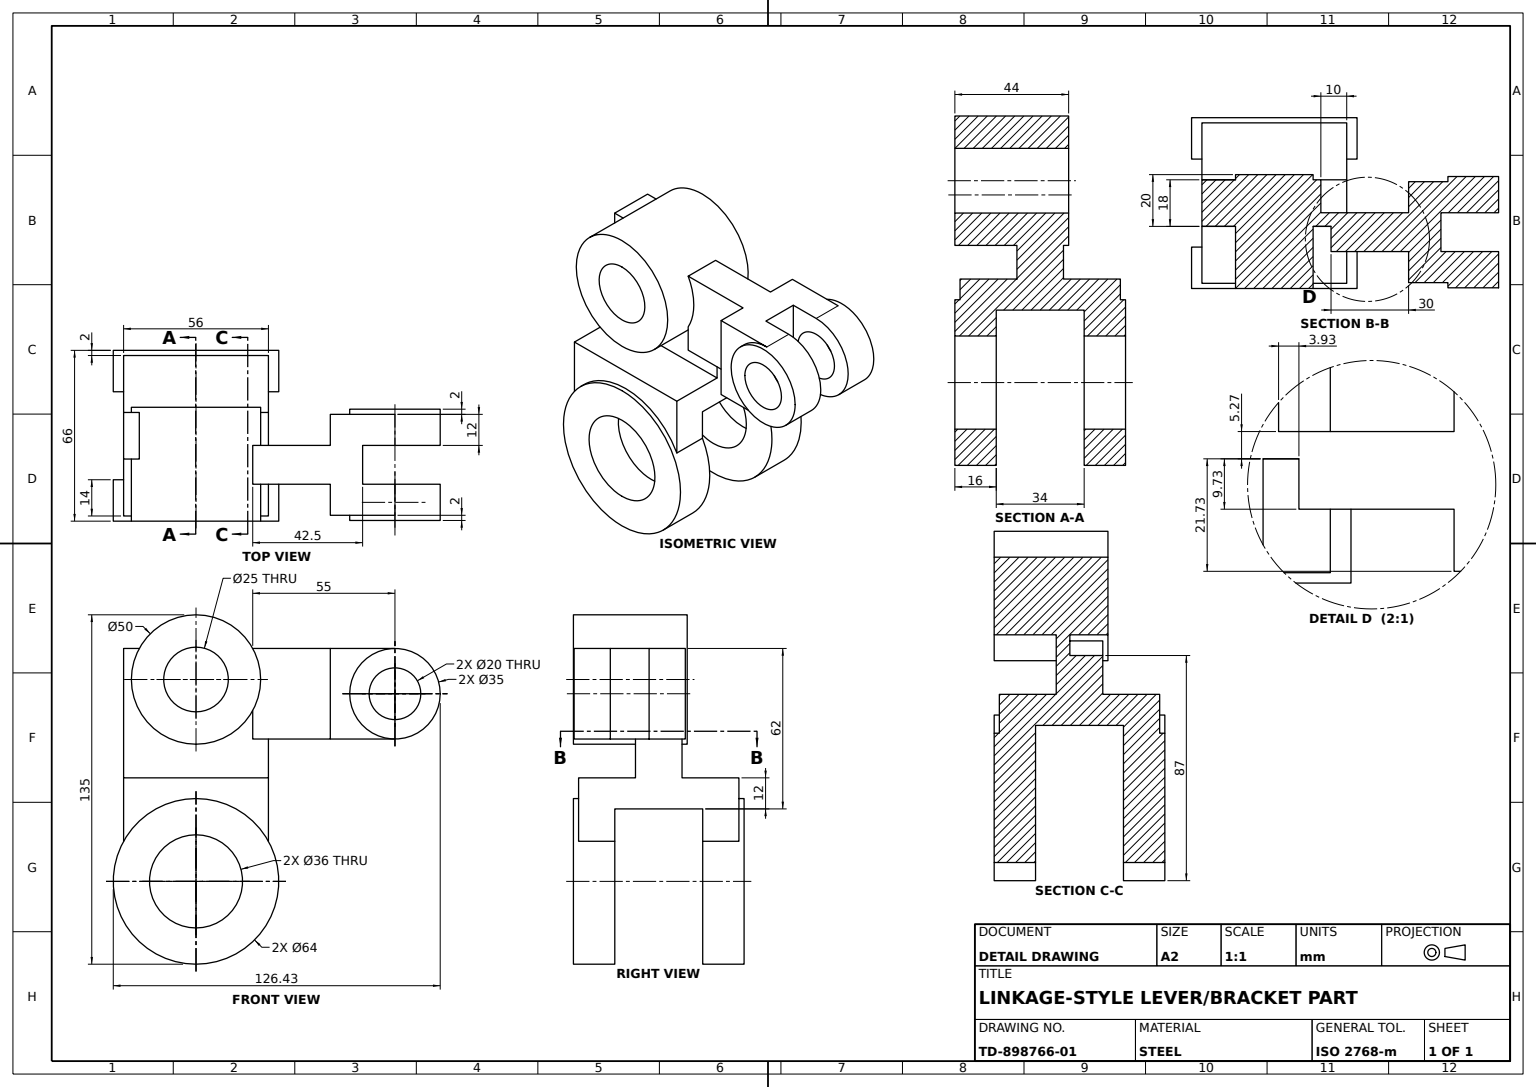
from build123d import *

# Parameters (mm, degrees)
BRACKET_BODY_DEPTH      = 56
SLOT_SKETCH_W           = 62
SLOT_SKETCH_H           = 20
SLOT_CUT_DEPTH          = 90.112288715
LUG_A_SKETCH_R          = 32
LUG_A_SKETCH_R_2        = 18
LUG_A_14MM_DEPTH        = 14
SPACER_START            = 2
SPACER_A_SKETCH_R       = 32
SPACER_A_SKETCH_R_2     = 18
SPACER_A_2MM_DEPTH      = 2
HOLE_A_SKETCH_R         = 18
HOLE_A_DEPTH            = 107.244999882
SPACER_B_SKETCH_R       = 32
SPACER_B_SKETCH_R_2     = 18
SPACER_B_2MM_DEPTH      = 2
LUG_B_SKETCH_R          = 32
LUG_B_SKETCH_R_2        = 18
LUG_B_14MM_DEPTH        = 14
PAD_SKETCH_R            = 25
PAD_SKETCH_R_2          = 12.5
PAD_2MM_DEPTH           = 2
HUB_START               = -44
HUB_SKETCH_R            = 25
HUB_SKETCH_R_2          = 12.5
HUB_44MM_DEPTH          = 44
HUB_BORE_SKETCH_R       = 12.5
HUB_BORE_DEPTH          = 44
ARM_35MM_DEPTH          = 35
ARM_SPACER_A_SKETCH_R   = 17.5
ARM_SPACER_A_SKETCH_R_2 = 10
ARM_SPACER_A_2MM_DEPTH  = 2
ARM_START               = -12
ARM_LUG_SKETCH_R        = 17.5
ARM_LUG_SKETCH_R_2      = 10
ARM_LUG_12MM_DEPTH      = 12
ARM_HOLE_SKETCH_R       = 10
ARM_HOLE_DEPTH          = 150.390672563
ARM_SPACER_B_SKETCH_R   = 17.5
ARM_SPACER_B_SKETCH_R_2 = 10
ARM_SPACER_B_2MM_DEPTH  = 2
ARM_START_2             = -14
ARM_EYE_SKETCH_R        = 17.5
ARM_EYE_SKETCH_R_2      = 10
ARM_EYE_14MM_DEPTH      = 14
ARM_SLOT_SKETCH_W       = 12.731987003
ARM_SLOT_SKETCH_H       = 35
ARM_SLOT_10MM_DEPTH     = 10
PIN_START               = -16
PIN_BOSS_SKETCH_R       = 25
PIN_BOSS_16MM_DEPTH     = 16
PIN_BOSS_HOLE_SKETCH_R  = 12.5
PIN_BOSS_HOLE_DEPTH     = 151.168319402


with BuildPart() as part:
    # Bracket Profile Sketch → Bracket Body (new body)
    with BuildSketch(Plane.XY):
        Polygon((0, 0), (17, 0), (17, -48), (31, -48), (31, 12), (9, 12), (9, 62), (-9, 62), (-9, 12), (-31, 12), (-31, -48), (-17, -48), (-17, 0), align=None)
    extrude(amount=-BRACKET_BODY_DEPTH)

    # Slot Sketch → Slot Cut (cut, through all)
    with BuildSketch(Plane.XY):
        with Locations((0, -38)):
            Rectangle(SLOT_SKETCH_W, SLOT_SKETCH_H)
    extrude(amount=-SLOT_CUT_DEPTH, mode=Mode.SUBTRACT)

    # Lug A Sketch → Lug A 14mm (add)
    with BuildSketch(Plane(origin=(31, 0, 0), x_dir=(0, 0, -1), z_dir=(1, 0, 0))):
        with Locations((28, -28)):
            Circle(LUG_A_SKETCH_R)
        with Locations((28, -28)):
            Circle(LUG_A_SKETCH_R_2, mode=Mode.SUBTRACT)
    extrude(amount=-LUG_A_14MM_DEPTH)

    # Spacer A Sketch → Spacer A 2mm (add)
    with BuildSketch(Plane(origin=(31, 0, 0), x_dir=(0, 0, -1), z_dir=(1, 0, 0)).offset(SPACER_START)):
        with Locations(Location((28, -28, 0), (0, 0, 90))):
            Circle(SPACER_A_SKETCH_R)
        with Locations(Location((28, -28, 0), (0, 0, 90))):
            Circle(SPACER_A_SKETCH_R_2, mode=Mode.SUBTRACT)
    extrude(amount=-SPACER_A_2MM_DEPTH)

    # Hole A Sketch → Hole A (cut, through all)
    with BuildSketch(Plane(origin=(31, 0, 0), x_dir=(0, 0, -1), z_dir=(1, 0, 0))):
        with Locations(Location((28, -28, 0), (0, 0, 90))):
            Circle(HOLE_A_SKETCH_R)
    extrude(amount=-HOLE_A_DEPTH, mode=Mode.SUBTRACT)

    # Spacer B Sketch → Spacer B 2mm (add)
    with BuildSketch(Plane.ZY.offset(31)):
        with Locations(Location((-28, -28, 0), (0, 0, 90))):
            Circle(SPACER_B_SKETCH_R)
        with Locations(Location((-28, -28, 0), (0, 0, 90))):
            Circle(SPACER_B_SKETCH_R_2, mode=Mode.SUBTRACT)
    extrude(amount=SPACER_B_2MM_DEPTH)

    # Lug B Sketch → Lug B 14mm (add)
    with BuildSketch(Plane(origin=(-17, 0, 0), x_dir=(0, 0, -1), z_dir=(1, 0, 0))):
        with Locations(Location((28, -28, 0), (0, 0, 90))):
            Circle(LUG_B_SKETCH_R)
        with Locations(Location((28, -28, 0), (0, 0, 90))):
            Circle(LUG_B_SKETCH_R_2, mode=Mode.SUBTRACT)
    extrude(amount=-LUG_B_14MM_DEPTH)

    # Pad Sketch → Pad 2mm (add)
    with BuildSketch(Plane.ZY.offset(9)):
        with Locations(Location((-28, 50, 0), (0, 0, 151.314597986))):
            Circle(PAD_SKETCH_R)
        with Locations(Location((-28, 50, 0), (0, 0, 73.739795292))):
            Circle(PAD_SKETCH_R_2, mode=Mode.SUBTRACT)
    extrude(amount=PAD_2MM_DEPTH)

    # Hub Sketch → Hub 44mm (add)
    with BuildSketch(Plane.ZY.offset(11).offset(HUB_START)):
        with Locations(Location((-28, 50, 0), (0, 0, 270))):
            Circle(HUB_SKETCH_R)
        with Locations(Location((-28, 50, 0), (0, 0, 270))):
            Circle(HUB_SKETCH_R_2, mode=Mode.SUBTRACT)
    extrude(amount=HUB_44MM_DEPTH)

    # Hub Bore Sketch → Hub Bore (cut)
    with BuildSketch(Plane.ZY.offset(9).offset(HUB_START)):
        with Locations(Location((-28, 50, 0), (0, 0, 270))):
            Circle(HUB_BORE_SKETCH_R)
    extrude(amount=HUB_BORE_DEPTH, mode=Mode.SUBTRACT)

    # Arm Profile Sketch → Arm 35mm (add)
    with BuildSketch(Plane(origin=(0, 62, 0), x_dir=(1, 0, 0), z_dir=(0, 1, 0))):
        Polygon((3.731987003, 49.931712199), (3.731987003, 79.931712199), (-8.268012997, 79.931712199), (-8.268012997, 104.931712199), (3.731987003, 104.931712199), (3.731987003, 92.431712199), (18.731987003, 92.431712199), (18.731987003, 104.931712199), (30.731987003, 104.931712199), (30.731987003, 79.931712199), (18.731987003, 79.931712199), (18.731987003, 49.931712199), align=None)
    extrude(amount=-ARM_35MM_DEPTH)

    # Arm Spacer A Sketch → Arm Spacer A 2mm (add)
    with BuildSketch(Plane.ZY.offset(8.268012997)):
        with Locations(Location((-104.931712199, 44.5, 0), (0, 0, 270))):
            Circle(ARM_SPACER_A_SKETCH_R)
        with Locations(Location((-104.931712199, 44.5, 0), (0, 0, 90))):
            Circle(ARM_SPACER_A_SKETCH_R_2, mode=Mode.SUBTRACT)
    extrude(amount=ARM_SPACER_A_2MM_DEPTH)

    # Arm Lug Sketch → Arm Lug 12mm (add)
    with BuildSketch(Plane.ZY.offset(8.268012997).offset(ARM_START)):
        with Locations(Location((-104.931712199, 44.5, 0), (0, 0, 90))):
            Circle(ARM_LUG_SKETCH_R)
        with Locations(Location((-104.931712199, 44.5, 0), (0, 0, 90))):
            Circle(ARM_LUG_SKETCH_R_2, mode=Mode.SUBTRACT)
    extrude(amount=ARM_LUG_12MM_DEPTH)

    # Arm Hole Sketch → Arm Hole (cut, through all)
    with BuildSketch(Plane.ZY.offset(8.268012997)):
        with Locations((-104.931712199, 44.5)):
            Circle(ARM_HOLE_SKETCH_R)
    extrude(amount=-ARM_HOLE_DEPTH, mode=Mode.SUBTRACT)

    # Arm Spacer B Sketch → Arm Spacer B 2mm (add)
    with BuildSketch(Plane(origin=(30.731987003, 0, 0), x_dir=(0, 0, -1), z_dir=(1, 0, 0))):
        with Locations(Location((104.931712199, 44.5, 0), (0, 0, 90))):
            Circle(ARM_SPACER_B_SKETCH_R)
        with Locations(Location((104.931712199, 44.5, 0), (0, 0, 180))):
            Circle(ARM_SPACER_B_SKETCH_R_2, mode=Mode.SUBTRACT)
    extrude(amount=ARM_SPACER_B_2MM_DEPTH)

    # Arm Eye Sketch → Arm Eye 14mm (add)
    with BuildSketch(Plane(origin=(32.731987003, 0, 0), x_dir=(0, 0, -1), z_dir=(1, 0, 0)).offset(ARM_START_2)):
        with Locations(Location((104.931712199, 44.5, 0), (0, 0, 90))):
            Circle(ARM_EYE_SKETCH_R)
        with Locations(Location((104.931712199, 44.5, 0), (0, 0, 180))):
            Circle(ARM_EYE_SKETCH_R_2, mode=Mode.SUBTRACT)
    extrude(amount=ARM_EYE_14MM_DEPTH)

    # Arm Slot Sketch → Arm Slot 10mm (cut)
    with BuildSketch(Plane(origin=(0, 0, -56), x_dir=(-1, 0, 0), z_dir=(0, 0, -1))):
        with Locations((2.634006498, 44.5)):
            Rectangle(ARM_SLOT_SKETCH_W, ARM_SLOT_SKETCH_H)
    extrude(amount=-ARM_SLOT_10MM_DEPTH, mode=Mode.SUBTRACT)

    # Pin Boss Sketch → Pin Boss 16mm (add)
    with BuildSketch(Plane.ZY.offset(11).offset(PIN_START)):
        with Locations(Location((-28, 50, 0), (0, 0, 270))):
            Circle(PIN_BOSS_SKETCH_R)
    extrude(amount=PIN_BOSS_16MM_DEPTH)

    # Pin Boss Hole Sketch → Pin Boss Hole (cut, through all)
    with BuildSketch(Plane.ZY.offset(11)):
        with Locations(Location((-28, 50, 0), (0, 0, 270))):
            Circle(PIN_BOSS_HOLE_SKETCH_R)
    extrude(amount=-PIN_BOSS_HOLE_DEPTH, mode=Mode.SUBTRACT)


solid = part.part
